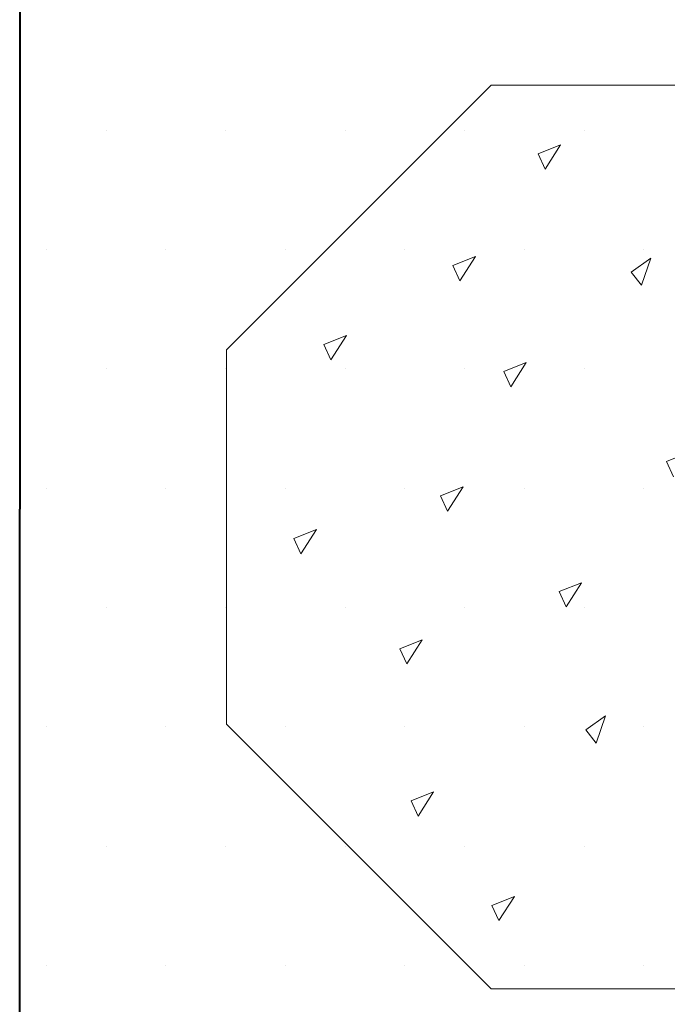
# Model space of a CAD drawing. Units: inches. Extents: x 459864 to 460310, y 324185 to 324787.
# Tile 4 of 112: x 460061.11 to 460069.72, y 324228.9 to 324241.99. Entities that reach past the tile are written whole.
import ezdxf

# ---------------------------------------------------------------- set-up
doc = ezdxf.new("R2010")
doc.units = ezdxf.units.IN
for name, color, linetype, lineweight in [('A-ANNO-DIMS', 2, 'Continuous', 18), ('A-WALL', 7, 'Continuous', 40), ('L-HRDS', 9, 'Continuous', 18), ('L-SITE-PATT', 252, 'Continuous', 13)]:
    doc.layers.add(name, color=color, linetype=linetype, lineweight=lineweight)
doc.styles.get("Standard").update_dxf_attribs({"font": 'arial.ttf'})
doc.dimstyles.new('ISO-25', dxfattribs={"dimtxt": 6, "dimasz": 2.5, "dimexe": 1.25, "dimexo": 0.625, "dimtad": 1, "dimdec": 1, "dimlunit": 3, "dimtxsty": 'Standard', "dimcen": 2.5, "dimadec": 0, "dimazin": 0, "dimtfac": 1, "dimtdec": 1, "dimtmove": 0, "dimatfit": 3, "dimfxl": 1, "dimarcsym": 0})

# ---------------------------------------------------------------- blocks, each defined once
blk = doc.blocks.new('Stepping Stone - hexagonal')
for p, q in [((-5.099, 10.067), (-10.964, 4.202)), ((3.195, 10.067), (-5.099, 10.067)), ((-3.564, 8.743), (-4.061, 8.544)), ((-3.906, 8.205), (-3.564, 8.743)), ((-4.061, 8.544), (-3.906, 8.205)), ((-5.451, 6.27), (-5.948, 6.072)), ((-5.793, 5.732), (-5.451, 6.27)), ((-1.567, 6.236), (-2.004, 5.927)), ((-1.775, 5.633), (-1.567, 6.236)), ((-5.948, 6.072), (-5.793, 5.732)), ((-2.004, 5.927), (-1.775, 5.633)), ((-8.308, 4.52), (-8.806, 4.321)), ((-8.651, 3.982), (-8.308, 4.52)), ((-10.964, 4.202), (-10.964, -4.092)), ((-8.806, 4.321), (-8.651, 3.982)), ((-4.324, 3.923), (-4.821, 3.724)), ((-4.821, 3.724), (-4.667, 3.385)), ((-4.667, 3.385), (-4.324, 3.923)), ((-0.723, 1.925), (-1.22, 1.726)), ((-1.22, 1.726), (-1.066, 1.387)), ((-5.724, 1.164), (-6.221, 0.965)), ((-6.066, 0.626), (-5.724, 1.164)), ((-6.221, 0.965), (-6.066, 0.626)), ((-8.972, 0.221), (-9.469, 0.023)), ((-9.314, -0.317), (-8.972, 0.221)), ((-9.469, 0.023), (-9.314, -0.317)), ((-3.099, -0.958), (-3.596, -1.157)), ((-3.441, -1.496), (-3.099, -0.958)), ((-3.596, -1.157), (-3.441, -1.496)), ((-6.63, -2.222), (-7.127, -2.421)), ((-6.972, -2.76), (-6.63, -2.222)), ((-7.127, -2.421), (-6.972, -2.76)), ((-2.567, -3.91), (-3.004, -4.219)), ((-2.774, -4.513), (-2.567, -3.91)), ((-10.964, -4.092), (-5.099, -9.957)), ((-3.004, -4.219), (-2.774, -4.513)), ((-6.377, -5.594), (-6.874, -5.792)), ((-6.719, -6.132), (-6.377, -5.594)), ((-6.874, -5.792), (-6.719, -6.132)), ((-4.588, -7.91), (-5.085, -8.109)), ((-4.93, -8.448), (-4.588, -7.91)), ((-5.085, -8.109), (-4.93, -8.448)), ((-5.099, -9.957), (3.195, -9.957))]:
    blk.add_line(p, q)
blk = doc.blocks.new('*D36')
at = {"layer": 'A-ANNO-DIMS', "color": 0, "lineweight": -2, "transparency": 16777216}
for p, q in [((460063.861, 324228.483), (460063.861, 324226.056)), ((460075.876, 324228.483), (460075.876, 324226.056)), ((460066.361, 324227.306), (460073.376, 324227.306)), ((460075.876, 324227.306), (460126.021, 324227.306))]:
    blk.add_line(p, q, dxfattribs=at)
at = {"layer": 'A-ANNO-DIMS', "color": 0, "transparency": 16777216}
for points in [[(460066.361, 324227.722), (460066.361, 324226.889), (460063.861, 324227.306)], [(460073.376, 324227.722), (460073.376, 324226.889), (460075.876, 324227.306)]]:
    blk.add_solid(points, dxfattribs=at)
at = {"layer": 'Defpoints', "color": 0, "transparency": 16777216}
for p in [(460063.861, 324229.108), (460075.876, 324229.108), (460075.876, 324227.306)]:
    blk.add_point(p, dxfattribs=at)
at = {"layer": 'A-ANNO-DIMS', "color": 0, "transparency": 16777216, "insert": (460102.199, 324230.994), "char_height": 6, "attachment_point": 5}
blk.add_mtext('PAVER 1\'-0"', dxfattribs=at)

msp = doc.modelspace()

# ---------------------------------------------------------------- hatches: boundary and pattern name
at = {"layer": 'L-SITE-PATT'}
h = msp.add_hatch(dxfattribs=at)
h.set_pattern_fill('DOTS', color=256)
h.paths.add_polyline_path([(460269.804, 324283.483), (460247.115, 324283.483), (460121.929, 324283.483), (460121.929, 324252.473), (460117.429, 324252.473), (460110.124, 324252.473), (460110.124, 324243.287), (460080.83, 324243.287), (460080.83, 324252.473), (460061.115, 324252.473), (460061.115, 324251.882), (460077.909, 324251.882), (460077.909, 324199.483), (460080.83, 324199.483), (460080.83, 324207.553), (460110.124, 324207.553), (460110.124, 324199.483), (460110.813, 324199.483), (460262.115, 324199.483), (460269.804, 324199.483)], flags=17)
edge = h.paths.add_edge_path(flags=0)
edge.add_ellipse((460222.59, 324263.813), major_axis=(-8.485, 8.485), ratio=1, start_angle=405, end_angle=495, ccw=False)
edge.add_line((460214.821, 324254.66), (460214.832, 324254.666))
edge.add_ellipse((460222.59, 324263.813), major_axis=(-8.485, 8.485), ratio=1, start_angle=405, end_angle=495, ccw=False)
edge.add_line((460210.759, 324261.781), (460210.768, 324261.787))
edge.add_ellipse((460222.59, 324263.813), major_axis=(-8.485, 8.485), ratio=1, start_angle=405, end_angle=495, ccw=False)
edge.add_ellipse((460222.59, 324263.813), major_axis=(-8.485, 8.485), ratio=1, start_angle=392.754, end_angle=405, ccw=False)
edge.add_ellipse((460222.59, 324263.813), major_axis=(-8.485, 8.485), ratio=1, start_angle=380.9347, end_angle=392.754, ccw=False)
edge.add_line((460211.337, 324267.985), (460211.34, 324267.985))
edge.add_ellipse((460222.59, 324263.813), major_axis=(-8.485, 8.485), ratio=1, start_angle=380.9347, end_angle=392.754, ccw=False)
edge.add_ellipse((460222.59, 324263.813), major_axis=(-8.485, 8.485), ratio=1, start_angle=347.9015, end_angle=380.9347, ccw=False)
edge.add_ellipse((460222.59, 324263.813), major_axis=(-8.485, 8.485), ratio=1, start_angle=327.0619, end_angle=347.9015, ccw=False)
edge.add_ellipse((460222.59, 324263.813), major_axis=(-8.485, 8.485), ratio=1, start_angle=278.3246, end_angle=327.0619, ccw=False)
edge.add_line((460225.158, 324275.536), (460225.158, 324275.535))
edge.add_ellipse((460222.59, 324263.813), major_axis=(-8.485, 8.485), ratio=1, start_angle=278.3246, end_angle=327.0619, ccw=False)
edge.add_ellipse((460222.59, 324263.813), major_axis=(-8.485, 8.485), ratio=1, start_angle=260.6436, end_angle=278.3246, ccw=False)
edge.add_ellipse((460222.59, 324263.813), major_axis=(-8.485, 8.485), ratio=1, start_angle=225, end_angle=260.6436, ccw=False)
edge.add_line((460234.509, 324265.243), (460234.501, 324265.239))
edge.add_ellipse((460222.59, 324263.813), major_axis=(-8.485, 8.485), ratio=1, start_angle=225, end_angle=260.6436, ccw=False)
edge.add_ellipse((460222.59, 324263.813), major_axis=(-8.485, 8.485), ratio=1, start_angle=495, end_angle=585, ccw=False)
edge.add_line((460234.437, 324261.861), (460234.424, 324261.858))
edge.add_ellipse((460222.59, 324263.813), major_axis=(-8.485, 8.485), ratio=1, start_angle=495, end_angle=585, ccw=False)
edge.add_line((460227.95, 324253.067), (460227.946, 324253.083))
edge.add_ellipse((460222.59, 324263.813), major_axis=(-8.485, 8.485), ratio=1, start_angle=495, end_angle=585, ccw=False)
edge.add_line((460226.223, 324252.369), (460226.211, 324252.38))
edge.add_ellipse((460222.59, 324263.813), major_axis=(-8.485, 8.485), ratio=1, start_angle=495, end_angle=585, ccw=False)
h.paths.add_polyline_path([(460219.651, 324254.347), (460218.461, 324253.545), (460218.275, 324254.789), (460219.642, 324256.542), (460219.625, 324260.848), (460216.11, 324257.333), (460214.35, 324256.978), (460215.416, 324259.356), (460212.524, 324258.496), (460213.137, 324259.93), (460218.507, 324263.813), (460222.59, 324263.813), (460222.59, 324267.807), (460218.176, 324272.212), (460219.026, 324274.639), (460222.59, 324272.811), (460222.59, 324275.423), (460223.057, 324274.825), (460222.675, 324273.492), (460225.912, 324267.135), (460219.625, 324260.848)], flags=0)
edge = h.paths.add_edge_path(flags=0)
edge.add_ellipse((460194.576, 324264.046), major_axis=(-8.485, 8.485), ratio=1, start_angle=495, end_angle=585, ccw=False)
edge.add_line((460199.936, 324253.3), (460199.932, 324253.316))
edge.add_ellipse((460194.576, 324264.046), major_axis=(-8.485, 8.485), ratio=1, start_angle=495, end_angle=585, ccw=False)
edge.add_line((460198.208, 324252.603), (460198.196, 324252.613))
edge.add_ellipse((460194.576, 324264.046), major_axis=(-8.485, 8.485), ratio=1, start_angle=495, end_angle=585, ccw=False)
edge.add_ellipse((460194.576, 324264.046), major_axis=(-8.485, 8.485), ratio=1, start_angle=405, end_angle=495, ccw=False)
edge.add_line((460186.806, 324254.893), (460186.817, 324254.899))
edge.add_ellipse((460194.576, 324264.046), major_axis=(-8.485, 8.485), ratio=1, start_angle=405, end_angle=495, ccw=False)
edge.add_line((460182.744, 324262.014), (460182.753, 324262.02))
edge.add_ellipse((460194.576, 324264.046), major_axis=(-8.485, 8.485), ratio=1, start_angle=405, end_angle=495, ccw=False)
edge.add_ellipse((460194.576, 324264.046), major_axis=(-8.485, 8.485), ratio=1, start_angle=392.754, end_angle=405, ccw=False)
edge.add_ellipse((460194.576, 324264.046), major_axis=(-8.485, 8.485), ratio=1, start_angle=380.9347, end_angle=392.754, ccw=False)
edge.add_line((460183.323, 324268.218), (460183.326, 324268.218))
edge.add_ellipse((460194.576, 324264.046), major_axis=(-8.485, 8.485), ratio=1, start_angle=380.9347, end_angle=392.754, ccw=False)
edge.add_ellipse((460194.576, 324264.046), major_axis=(-8.485, 8.485), ratio=1, start_angle=347.9015, end_angle=380.9347, ccw=False)
edge.add_ellipse((460194.576, 324264.046), major_axis=(-8.485, 8.485), ratio=1, start_angle=327.0619, end_angle=347.9015, ccw=False)
edge.add_ellipse((460194.576, 324264.046), major_axis=(-8.485, 8.485), ratio=1, start_angle=278.3246, end_angle=327.0619, ccw=False)
edge.add_line((460197.144, 324275.769), (460197.143, 324275.768))
edge.add_ellipse((460194.576, 324264.046), major_axis=(-8.485, 8.485), ratio=1, start_angle=278.3246, end_angle=327.0619, ccw=False)
edge.add_ellipse((460194.576, 324264.046), major_axis=(-8.485, 8.485), ratio=1, start_angle=260.6436, end_angle=278.3246, ccw=False)
edge.add_ellipse((460194.576, 324264.046), major_axis=(-8.485, 8.485), ratio=1, start_angle=225, end_angle=260.6436, ccw=False)
edge.add_line((460206.494, 324265.476), (460206.487, 324265.473))
edge.add_ellipse((460194.576, 324264.046), major_axis=(-8.485, 8.485), ratio=1, start_angle=225, end_angle=260.6436, ccw=False)
edge.add_ellipse((460194.576, 324264.046), major_axis=(-8.485, 8.485), ratio=1, start_angle=495, end_angle=585, ccw=False)
edge.add_line((460206.422, 324262.094), (460206.409, 324262.091))
h.paths.add_polyline_path([(460191.61, 324261.081), (460191.637, 324254.58), (460190.447, 324253.778), (460190.261, 324255.023), (460191.628, 324256.775), (460191.61, 324261.081), (460188.096, 324257.566), (460186.335, 324257.211), (460187.402, 324259.589), (460184.509, 324258.729), (460185.123, 324260.163), (460190.493, 324264.046), (460194.576, 324264.046), (460194.576, 324268.04), (460190.161, 324272.446), (460191.011, 324274.872), (460194.576, 324273.044), (460194.576, 324275.657), (460195.043, 324275.058), (460194.661, 324273.725), (460197.897, 324267.368)], flags=0)
edge = h.paths.add_edge_path(flags=0)
edge.add_ellipse((460252.912, 324263.578), major_axis=(-8.485, 8.485), ratio=1, start_angle=405, end_angle=495, ccw=False)
edge.add_line((460241.081, 324261.545), (460241.089, 324261.551))
edge.add_ellipse((460252.912, 324263.578), major_axis=(-8.485, 8.485), ratio=1, start_angle=405, end_angle=495, ccw=False)
edge.add_ellipse((460252.912, 324263.578), major_axis=(-8.485, 8.485), ratio=1, start_angle=392.754, end_angle=405, ccw=False)
edge.add_ellipse((460252.912, 324263.578), major_axis=(-8.485, 8.485), ratio=1, start_angle=380.9347, end_angle=392.754, ccw=False)
edge.add_line((460241.659, 324267.749), (460241.662, 324267.749))
edge.add_ellipse((460252.912, 324263.578), major_axis=(-8.485, 8.485), ratio=1, start_angle=380.9347, end_angle=392.754, ccw=False)
edge.add_ellipse((460252.912, 324263.578), major_axis=(-8.485, 8.485), ratio=1, start_angle=347.9015, end_angle=380.9347, ccw=False)
edge.add_ellipse((460252.912, 324263.578), major_axis=(-8.485, 8.485), ratio=1, start_angle=327.0619, end_angle=347.9015, ccw=False)
edge.add_ellipse((460252.912, 324263.578), major_axis=(-8.485, 8.485), ratio=1, start_angle=278.3246, end_angle=327.0619, ccw=False)
edge.add_line((460255.48, 324275.3), (460255.479, 324275.299))
edge.add_ellipse((460252.912, 324263.578), major_axis=(-8.485, 8.485), ratio=1, start_angle=278.3246, end_angle=327.0619, ccw=False)
edge.add_ellipse((460252.912, 324263.578), major_axis=(-8.485, 8.485), ratio=1, start_angle=260.6436, end_angle=278.3246, ccw=False)
edge.add_ellipse((460252.912, 324263.578), major_axis=(-8.485, 8.485), ratio=1, start_angle=225, end_angle=260.6436, ccw=False)
edge.add_line((460264.83, 324265.007), (460264.823, 324265.004))
edge.add_ellipse((460252.912, 324263.578), major_axis=(-8.485, 8.485), ratio=1, start_angle=225, end_angle=260.6436, ccw=False)
edge.add_ellipse((460252.912, 324263.578), major_axis=(-8.485, 8.485), ratio=1, start_angle=495, end_angle=585, ccw=False)
edge.add_line((460264.758, 324261.626), (460264.745, 324261.622))
edge.add_ellipse((460252.912, 324263.578), major_axis=(-8.485, 8.485), ratio=1, start_angle=495, end_angle=585, ccw=False)
edge.add_line((460258.272, 324252.832), (460258.268, 324252.848))
edge.add_ellipse((460252.912, 324263.578), major_axis=(-8.485, 8.485), ratio=1, start_angle=495, end_angle=585, ccw=False)
edge.add_line((460256.545, 324252.134), (460256.533, 324252.144))
edge.add_ellipse((460252.912, 324263.578), major_axis=(-8.485, 8.485), ratio=1, start_angle=495, end_angle=585, ccw=False)
edge.add_ellipse((460252.912, 324263.578), major_axis=(-8.485, 8.485), ratio=1, start_angle=405, end_angle=495, ccw=False)
edge.add_line((460245.143, 324254.424), (460245.153, 324254.43))
h.paths.add_polyline_path([(460244.672, 324256.742), (460245.738, 324259.12), (460242.846, 324258.26), (460243.459, 324259.694), (460248.829, 324263.578), (460252.912, 324263.578), (460252.912, 324267.571), (460248.497, 324271.977), (460249.348, 324274.403), (460252.912, 324272.576), (460252.912, 324275.188), (460253.379, 324274.589), (460252.997, 324273.257), (460256.233, 324266.899), (460249.946, 324260.612), (460249.973, 324254.111), (460248.783, 324253.309), (460248.597, 324254.554), (460249.964, 324256.306), (460249.946, 324260.612), (460246.432, 324257.097)], flags=0)
edge = h.paths.add_edge_path(flags=0)
edge.add_ellipse((460167.439, 324262.833), major_axis=(-8.485, 8.485), ratio=1, start_angle=495, end_angle=585, ccw=False)
edge.add_line((460172.799, 324252.087), (460172.795, 324252.103))
edge.add_ellipse((460167.439, 324262.833), major_axis=(-8.485, 8.485), ratio=1, start_angle=495, end_angle=585, ccw=False)
edge.add_line((460171.071, 324251.389), (460171.059, 324251.399))
edge.add_ellipse((460167.439, 324262.833), major_axis=(-8.485, 8.485), ratio=1, start_angle=495, end_angle=585, ccw=False)
edge.add_ellipse((460167.439, 324262.833), major_axis=(-8.485, 8.485), ratio=1, start_angle=405, end_angle=495, ccw=False)
edge.add_line((460159.669, 324253.679), (460159.68, 324253.685))
edge.add_ellipse((460167.439, 324262.833), major_axis=(-8.485, 8.485), ratio=1, start_angle=405, end_angle=495, ccw=False)
edge.add_line((460155.607, 324260.8), (460155.616, 324260.806))
edge.add_ellipse((460167.439, 324262.833), major_axis=(-8.485, 8.485), ratio=1, start_angle=405, end_angle=495, ccw=False)
edge.add_ellipse((460167.439, 324262.833), major_axis=(-8.485, 8.485), ratio=1, start_angle=392.754, end_angle=405, ccw=False)
edge.add_ellipse((460167.439, 324262.833), major_axis=(-8.485, 8.485), ratio=1, start_angle=380.9347, end_angle=392.754, ccw=False)
edge.add_line((460156.185, 324267.005), (460156.189, 324267.005))
edge.add_ellipse((460167.439, 324262.833), major_axis=(-8.485, 8.485), ratio=1, start_angle=380.9347, end_angle=392.754, ccw=False)
edge.add_ellipse((460167.439, 324262.833), major_axis=(-8.485, 8.485), ratio=1, start_angle=347.9015, end_angle=380.9347, ccw=False)
edge.add_ellipse((460167.439, 324262.833), major_axis=(-8.485, 8.485), ratio=1, start_angle=327.0619, end_angle=347.9015, ccw=False)
edge.add_ellipse((460167.439, 324262.833), major_axis=(-8.485, 8.485), ratio=1, start_angle=278.3246, end_angle=327.0619, ccw=False)
edge.add_line((460170.007, 324274.556), (460170.006, 324274.554))
edge.add_ellipse((460167.439, 324262.833), major_axis=(-8.485, 8.485), ratio=1, start_angle=278.3246, end_angle=327.0619, ccw=False)
edge.add_ellipse((460167.439, 324262.833), major_axis=(-8.485, 8.485), ratio=1, start_angle=260.6436, end_angle=278.3246, ccw=False)
edge.add_ellipse((460167.439, 324262.833), major_axis=(-8.485, 8.485), ratio=1, start_angle=225, end_angle=260.6436, ccw=False)
edge.add_line((460179.357, 324264.262), (460179.35, 324264.259))
edge.add_ellipse((460167.439, 324262.833), major_axis=(-8.485, 8.485), ratio=1, start_angle=225, end_angle=260.6436, ccw=False)
edge.add_ellipse((460167.439, 324262.833), major_axis=(-8.485, 8.485), ratio=1, start_angle=495, end_angle=585, ccw=False)
edge.add_line((460179.285, 324260.881), (460179.272, 324260.877))
h.paths.add_polyline_path([(460164.473, 324259.867), (460164.5, 324253.366), (460163.31, 324252.565), (460163.124, 324253.809), (460164.491, 324255.561), (460164.473, 324259.867), (460160.958, 324256.353), (460159.198, 324255.998), (460160.265, 324258.375), (460157.372, 324257.515), (460157.986, 324258.949), (460163.356, 324262.833), (460167.439, 324262.833), (460167.439, 324266.826), (460163.024, 324271.232), (460163.874, 324273.659), (460167.439, 324271.831), (460167.439, 324274.443), (460167.905, 324273.844), (460167.524, 324272.512), (460170.76, 324266.154)], flags=0)
edge = h.paths.add_edge_path(flags=0)
edge.add_ellipse((460140.758, 324262.37), major_axis=(-8.485, 8.485), ratio=1, start_angle=495, end_angle=585, ccw=False)
edge.add_line((460146.118, 324251.624), (460146.114, 324251.639))
edge.add_ellipse((460140.758, 324262.37), major_axis=(-8.485, 8.485), ratio=1, start_angle=495, end_angle=585, ccw=False)
edge.add_line((460144.391, 324250.926), (460144.379, 324250.936))
edge.add_ellipse((460140.758, 324262.37), major_axis=(-8.485, 8.485), ratio=1, start_angle=495, end_angle=585, ccw=False)
edge.add_ellipse((460140.758, 324262.37), major_axis=(-8.485, 8.485), ratio=1, start_angle=405, end_angle=495, ccw=False)
edge.add_line((460132.989, 324253.216), (460132.999, 324253.222))
edge.add_ellipse((460140.758, 324262.37), major_axis=(-8.485, 8.485), ratio=1, start_angle=405, end_angle=495, ccw=False)
edge.add_line((460128.927, 324260.337), (460128.935, 324260.343))
edge.add_ellipse((460140.758, 324262.37), major_axis=(-8.485, 8.485), ratio=1, start_angle=405, end_angle=495, ccw=False)
edge.add_ellipse((460140.758, 324262.37), major_axis=(-8.485, 8.485), ratio=1, start_angle=392.754, end_angle=405, ccw=False)
edge.add_ellipse((460140.758, 324262.37), major_axis=(-8.485, 8.485), ratio=1, start_angle=380.9347, end_angle=392.754, ccw=False)
edge.add_line((460129.505, 324266.541), (460129.508, 324266.541))
edge.add_ellipse((460140.758, 324262.37), major_axis=(-8.485, 8.485), ratio=1, start_angle=380.9347, end_angle=392.754, ccw=False)
edge.add_ellipse((460140.758, 324262.37), major_axis=(-8.485, 8.485), ratio=1, start_angle=347.9015, end_angle=380.9347, ccw=False)
edge.add_ellipse((460140.758, 324262.37), major_axis=(-8.485, 8.485), ratio=1, start_angle=327.0619, end_angle=347.9015, ccw=False)
edge.add_ellipse((460140.758, 324262.37), major_axis=(-8.485, 8.485), ratio=1, start_angle=278.3246, end_angle=327.0619, ccw=False)
edge.add_line((460143.326, 324274.092), (460143.325, 324274.091))
edge.add_ellipse((460140.758, 324262.37), major_axis=(-8.485, 8.485), ratio=1, start_angle=278.3246, end_angle=327.0619, ccw=False)
edge.add_ellipse((460140.758, 324262.37), major_axis=(-8.485, 8.485), ratio=1, start_angle=260.6436, end_angle=278.3246, ccw=False)
edge.add_ellipse((460140.758, 324262.37), major_axis=(-8.485, 8.485), ratio=1, start_angle=225, end_angle=260.6436, ccw=False)
edge.add_line((460152.677, 324263.799), (460152.669, 324263.796))
edge.add_ellipse((460140.758, 324262.37), major_axis=(-8.485, 8.485), ratio=1, start_angle=225, end_angle=260.6436, ccw=False)
edge.add_ellipse((460140.758, 324262.37), major_axis=(-8.485, 8.485), ratio=1, start_angle=495, end_angle=585, ccw=False)
edge.add_line((460152.604, 324260.418), (460152.592, 324260.414))
h.paths.add_polyline_path([(460137.792, 324259.404), (460137.819, 324252.903), (460136.629, 324252.101), (460136.443, 324253.346), (460137.81, 324255.098), (460137.792, 324259.404), (460134.278, 324255.889), (460132.518, 324255.534), (460133.584, 324257.912), (460130.692, 324257.052), (460131.305, 324258.486), (460136.675, 324262.37), (460140.758, 324262.37), (460140.758, 324266.363), (460136.343, 324270.769), (460137.194, 324273.195), (460140.758, 324271.367), (460140.758, 324273.98), (460141.225, 324273.381), (460140.843, 324272.049), (460144.079, 324265.691)], flags=0)
h.paths.add_polyline_path([(460110.124, 324227.414), (460080.83, 324227.414), (460080.83, 324235.484), (460110.124, 324235.484)], flags=16)
h.paths.add_polyline_path([(460110.124, 324220.797), (460110.124, 324212.727), (460080.83, 324212.727), (460080.83, 324220.797)], flags=16)
h.paths.add_polyline_path([(460269.804, 324283.483), (460247.115, 324283.483), (460121.929, 324283.483), (460121.929, 324252.473), (460117.429, 324252.473), (460110.124, 324252.473), (460110.124, 324243.287), (460080.83, 324243.287), (460080.83, 324252.473), (460061.115, 324252.473), (460061.115, 324251.882), (460077.909, 324251.882), (460077.909, 324199.483), (460080.83, 324199.483), (460080.83, 324207.553), (460110.124, 324207.553), (460110.124, 324199.483), (460262.115, 324199.483), (460269.804, 324199.483)], flags=17)
h.paths.add_polyline_path([(460219.651, 324254.347), (460218.461, 324253.545), (460218.275, 324254.789), (460219.642, 324256.542), (460219.625, 324260.848), (460216.11, 324257.333), (460214.35, 324256.978), (460215.416, 324259.356), (460212.524, 324258.496), (460213.137, 324259.93), (460218.507, 324263.813), (460222.59, 324263.813), (460220.18, 324266.223), (460215.461, 324265.308), (460211.835, 324266.137), (460216.247, 324267.985), (460218.418, 324267.985), (460222.59, 324263.813), (460222.59, 324267.807), (460218.176, 324272.212), (460219.026, 324274.639), (460222.59, 324272.811), (460222.59, 324275.423), (460223.057, 324274.825), (460222.675, 324273.492), (460225.912, 324267.135), (460222.59, 324263.813), (460231.383, 324263.813), (460228.485, 324262.488), (460224.425, 324261.978), (460228.68, 324257.724), (460228.966, 324254.791), (460227.142, 324256.537), (460227.542, 324254.819), (460227.333, 324253.614), (460222.59, 324259.985), (460222.59, 324255.497), (460221.377, 324256.541), (460220.576, 324261.799), (460219.625, 324260.848)], flags=0)
h.paths.add_polyline_path([(460199.127, 324256.77), (460199.528, 324255.052), (460199.319, 324253.848), (460194.576, 324260.218), (460194.576, 324255.73), (460193.363, 324256.774), (460192.561, 324262.032), (460191.61, 324261.081), (460191.637, 324254.58), (460190.447, 324253.778), (460190.261, 324255.023), (460191.628, 324256.775), (460191.61, 324261.081), (460188.096, 324257.566), (460186.335, 324257.211), (460187.402, 324259.589), (460184.509, 324258.729), (460185.123, 324260.163), (460190.493, 324264.046), (460194.576, 324264.046), (460192.166, 324266.456), (460187.446, 324265.541), (460183.82, 324266.37), (460188.232, 324268.218), (460190.404, 324268.218), (460194.576, 324264.046), (460194.576, 324268.04), (460190.161, 324272.446), (460191.011, 324274.872), (460194.576, 324273.044), (460194.576, 324275.657), (460195.043, 324275.058), (460194.661, 324273.725), (460197.897, 324267.368), (460194.576, 324264.046), (460203.368, 324264.046), (460200.47, 324262.721), (460196.411, 324262.212), (460200.665, 324257.957), (460200.951, 324255.024)], flags=0)
h.paths.add_polyline_path([(460244.672, 324256.742), (460245.738, 324259.12), (460242.846, 324258.26), (460243.459, 324259.694), (460248.829, 324263.578), (460252.912, 324263.578), (460250.502, 324265.987), (460245.783, 324265.072), (460242.156, 324265.901), (460246.568, 324267.749), (460248.74, 324267.749), (460252.912, 324263.578), (460252.912, 324267.571), (460248.497, 324271.977), (460249.348, 324274.403), (460252.912, 324272.576), (460252.912, 324275.188), (460253.379, 324274.589), (460252.997, 324273.257), (460256.233, 324266.899), (460252.912, 324263.578), (460261.705, 324263.578), (460258.806, 324262.252), (460254.747, 324261.743), (460259.002, 324257.488), (460259.288, 324254.555), (460257.463, 324256.301), (460257.864, 324254.583), (460257.655, 324253.379), (460252.912, 324259.749), (460252.912, 324255.261), (460251.699, 324256.305), (460250.897, 324261.563), (460249.946, 324260.612), (460249.973, 324254.111), (460248.783, 324253.309), (460248.597, 324254.554), (460249.964, 324256.306), (460249.946, 324260.612), (460246.432, 324257.097)], flags=0)
h.paths.add_polyline_path([(460173.528, 324256.743), (460173.814, 324253.811), (460171.99, 324255.556), (460172.39, 324253.838), (460172.182, 324252.634), (460167.439, 324259.004), (460167.439, 324254.516), (460166.226, 324255.56), (460165.424, 324260.818), (460164.473, 324259.867), (460164.5, 324253.366), (460163.31, 324252.565), (460163.124, 324253.809), (460164.491, 324255.561), (460164.473, 324259.867), (460160.958, 324256.353), (460159.198, 324255.998), (460160.265, 324258.375), (460157.372, 324257.515), (460157.986, 324258.949), (460163.356, 324262.833), (460167.439, 324262.833), (460165.029, 324265.243), (460160.309, 324264.327), (460156.683, 324265.156), (460161.095, 324267.005), (460163.267, 324267.005), (460167.439, 324262.833), (460167.439, 324266.826), (460163.024, 324271.232), (460163.874, 324273.659), (460167.439, 324271.831), (460167.439, 324274.443), (460167.905, 324273.844), (460167.524, 324272.512), (460170.76, 324266.154), (460167.439, 324262.833), (460176.231, 324262.833), (460173.333, 324261.507), (460169.274, 324260.998)], flags=0)
h.paths.add_polyline_path([(460146.848, 324256.28), (460147.134, 324253.347), (460145.31, 324255.093), (460145.71, 324253.375), (460145.501, 324252.171), (460140.758, 324258.541), (460140.758, 324254.053), (460139.545, 324255.097), (460138.744, 324260.355), (460137.792, 324259.404), (460137.819, 324252.903), (460136.629, 324252.101), (460136.443, 324253.346), (460137.81, 324255.098), (460137.792, 324259.404), (460134.278, 324255.889), (460132.518, 324255.534), (460133.584, 324257.912), (460130.692, 324257.052), (460131.305, 324258.486), (460136.675, 324262.37), (460140.758, 324262.37), (460138.348, 324264.779), (460133.629, 324263.864), (460130.002, 324264.693), (460134.414, 324266.541), (460136.586, 324266.541), (460140.758, 324262.37), (460140.758, 324266.363), (460136.343, 324270.769), (460137.194, 324273.195), (460140.758, 324271.367), (460140.758, 324273.98), (460141.225, 324273.381), (460140.843, 324272.049), (460144.079, 324265.691), (460140.758, 324262.37), (460149.551, 324262.37), (460146.653, 324261.044), (460142.593, 324260.535)], flags=0)
edge = h.paths.add_edge_path()
edge.add_line((460269.804, 324272.549), (460260.881, 324272.549))
edge.add_ellipse((460252.912, 324263.578), major_axis=(-8.485, 8.485), ratio=1, start_angle=260.6436, end_angle=273.3846, ccw=False)
edge.add_line((460262.283, 324271.092), (460262.261, 324271.091))
edge.add_ellipse((460252.912, 324263.578), major_axis=(-8.485, 8.485), ratio=1, start_angle=260.6436, end_angle=273.3846, ccw=False)
edge.add_ellipse((460252.912, 324263.578), major_axis=(-8.485, 8.485), ratio=1, start_angle=225, end_angle=260.6436, ccw=False)
edge.add_line((460263.609, 324269.063), (460263.572, 324269.058))
edge.add_ellipse((460252.912, 324263.578), major_axis=(-8.485, 8.485), ratio=1, start_angle=225, end_angle=260.6436, ccw=False)
edge.add_line((460264.615, 324266.306), (460264.585, 324266.305))
edge.add_ellipse((460252.912, 324263.578), major_axis=(-8.485, 8.485), ratio=1, start_angle=225, end_angle=260.6436, ccw=False)
edge.add_line((460264.83, 324265.007), (460264.823, 324265.004))
edge.add_ellipse((460252.912, 324263.578), major_axis=(-8.485, 8.485), ratio=1, start_angle=225, end_angle=260.6436, ccw=False)
edge.add_ellipse((460252.912, 324263.578), major_axis=(-8.485, 8.485), ratio=1, start_angle=495, end_angle=585, ccw=False)
edge.add_line((460264.758, 324261.626), (460264.745, 324261.622))
edge.add_ellipse((460252.912, 324263.578), major_axis=(-8.485, 8.485), ratio=1, start_angle=495, end_angle=585, ccw=False)
edge.add_line((460263.442, 324257.739), (460263.389, 324257.779))
edge.add_ellipse((460252.912, 324263.578), major_axis=(-8.485, 8.485), ratio=1, start_angle=495, end_angle=585, ccw=False)
edge.add_line((460258.128, 324252.744), (460258.102, 324252.779))
edge.add_ellipse((460252.912, 324263.578), major_axis=(-8.485, 8.485), ratio=1, start_angle=495, end_angle=585, ccw=False)
edge.add_line((460256.545, 324252.134), (460256.533, 324252.144))
edge.add_ellipse((460252.912, 324263.578), major_axis=(-8.485, 8.485), ratio=1, start_angle=495, end_angle=585, ccw=False)
edge.add_ellipse((460252.912, 324263.578), major_axis=(-8.485, 8.485), ratio=1, start_angle=405, end_angle=495, ccw=False)
edge.add_line((460250.594, 324251.78), (460250.605, 324251.82))
edge.add_ellipse((460252.912, 324263.578), major_axis=(-8.485, 8.485), ratio=1, start_angle=405, end_angle=495, ccw=False)
edge.add_line((460245.143, 324254.424), (460245.153, 324254.43))
edge.add_ellipse((460252.912, 324263.578), major_axis=(-8.485, 8.485), ratio=1, start_angle=405, end_angle=495, ccw=False)
edge.add_line((460243.525, 324256.059), (460243.56, 324256.091))
edge.add_ellipse((460252.912, 324263.578), major_axis=(-8.485, 8.485), ratio=1, start_angle=405, end_angle=495, ccw=False)
edge.add_line((460241.44, 324259.893), (460241.522, 324259.896))
edge.add_ellipse((460252.912, 324263.578), major_axis=(-8.485, 8.485), ratio=1, start_angle=405, end_angle=495, ccw=False)
edge.add_line((460241.081, 324261.545), (460241.089, 324261.551))
edge.add_ellipse((460252.912, 324263.578), major_axis=(-8.485, 8.485), ratio=1, start_angle=405, end_angle=495, ccw=False)
edge.add_ellipse((460252.912, 324263.578), major_axis=(-8.485, 8.485), ratio=1, start_angle=392.754, end_angle=405, ccw=False)
edge.add_line((460241.05, 324265.438), (460241.063, 324265.443))
edge.add_ellipse((460252.912, 324263.578), major_axis=(-8.485, 8.485), ratio=1, start_angle=392.754, end_angle=405, ccw=False)
edge.add_ellipse((460252.912, 324263.578), major_axis=(-8.485, 8.485), ratio=1, start_angle=380.9347, end_angle=392.754, ccw=False)
edge.add_line((460241.452, 324267.176), (460241.469, 324267.171))
edge.add_ellipse((460252.912, 324263.578), major_axis=(-8.485, 8.485), ratio=1, start_angle=380.9347, end_angle=392.754, ccw=False)
edge.add_line((460241.659, 324267.749), (460241.662, 324267.749))
edge.add_ellipse((460252.912, 324263.578), major_axis=(-8.485, 8.485), ratio=1, start_angle=380.9347, end_angle=392.754, ccw=False)
edge.add_ellipse((460252.912, 324263.578), major_axis=(-8.485, 8.485), ratio=1, start_angle=356.6154, end_angle=380.9347, ccw=False)
edge.add_line((460244.88, 324272.488), (460244.713, 324272.549))
edge.add_line((460244.713, 324272.549), (460230.817, 324272.549))
edge.add_ellipse((460222.59, 324263.813), major_axis=(-8.485, 8.485), ratio=1, start_angle=260.6436, end_angle=271.7178, ccw=False)
edge.add_ellipse((460222.59, 324263.813), major_axis=(-8.485, 8.485), ratio=1, start_angle=225, end_angle=260.6436, ccw=False)
edge.add_line((460233.287, 324269.299), (460233.25, 324269.294))
edge.add_ellipse((460222.59, 324263.813), major_axis=(-8.485, 8.485), ratio=1, start_angle=225, end_angle=260.6436, ccw=False)
edge.add_line((460234.294, 324266.541), (460234.264, 324266.541))
edge.add_ellipse((460222.59, 324263.813), major_axis=(-8.485, 8.485), ratio=1, start_angle=225, end_angle=260.6436, ccw=False)
edge.add_line((460234.509, 324265.243), (460234.501, 324265.239))
edge.add_ellipse((460222.59, 324263.813), major_axis=(-8.485, 8.485), ratio=1, start_angle=225, end_angle=260.6436, ccw=False)
edge.add_ellipse((460222.59, 324263.813), major_axis=(-8.485, 8.485), ratio=1, start_angle=495, end_angle=585, ccw=False)
edge.add_line((460234.437, 324261.861), (460234.424, 324261.858))
edge.add_ellipse((460222.59, 324263.813), major_axis=(-8.485, 8.485), ratio=1, start_angle=495, end_angle=585, ccw=False)
edge.add_line((460233.121, 324257.975), (460233.068, 324258.015))
edge.add_ellipse((460222.59, 324263.813), major_axis=(-8.485, 8.485), ratio=1, start_angle=495, end_angle=585, ccw=False)
edge.add_line((460227.806, 324252.979), (460227.78, 324253.014))
edge.add_ellipse((460222.59, 324263.813), major_axis=(-8.485, 8.485), ratio=1, start_angle=495, end_angle=585, ccw=False)
edge.add_line((460226.223, 324252.369), (460226.211, 324252.38))
edge.add_ellipse((460222.59, 324263.813), major_axis=(-8.485, 8.485), ratio=1, start_angle=495, end_angle=585, ccw=False)
edge.add_ellipse((460222.59, 324263.813), major_axis=(-8.485, 8.485), ratio=1, start_angle=405, end_angle=495, ccw=False)
edge.add_line((460220.272, 324252.016), (460220.283, 324252.055))
edge.add_ellipse((460222.59, 324263.813), major_axis=(-8.485, 8.485), ratio=1, start_angle=405, end_angle=495, ccw=False)
edge.add_line((460214.821, 324254.66), (460214.832, 324254.666))
edge.add_ellipse((460222.59, 324263.813), major_axis=(-8.485, 8.485), ratio=1, start_angle=405, end_angle=495, ccw=False)
edge.add_line((460213.203, 324256.295), (460213.239, 324256.327))
edge.add_ellipse((460222.59, 324263.813), major_axis=(-8.485, 8.485), ratio=1, start_angle=405, end_angle=495, ccw=False)
edge.add_line((460211.118, 324260.128), (460211.201, 324260.131))
edge.add_ellipse((460222.59, 324263.813), major_axis=(-8.485, 8.485), ratio=1, start_angle=405, end_angle=495, ccw=False)
edge.add_line((460210.759, 324261.781), (460210.768, 324261.787))
edge.add_ellipse((460222.59, 324263.813), major_axis=(-8.485, 8.485), ratio=1, start_angle=405, end_angle=495, ccw=False)
edge.add_ellipse((460222.59, 324263.813), major_axis=(-8.485, 8.485), ratio=1, start_angle=392.754, end_angle=405, ccw=False)
edge.add_line((460210.729, 324265.673), (460210.741, 324265.678))
edge.add_ellipse((460222.59, 324263.813), major_axis=(-8.485, 8.485), ratio=1, start_angle=392.754, end_angle=405, ccw=False)
edge.add_ellipse((460222.59, 324263.813), major_axis=(-8.485, 8.485), ratio=1, start_angle=380.9347, end_angle=392.754, ccw=False)
edge.add_line((460211.13, 324267.412), (460211.147, 324267.407))
edge.add_ellipse((460222.59, 324263.813), major_axis=(-8.485, 8.485), ratio=1, start_angle=380.9347, end_angle=392.754, ccw=False)
edge.add_line((460211.337, 324267.985), (460211.34, 324267.985))
edge.add_ellipse((460222.59, 324263.813), major_axis=(-8.485, 8.485), ratio=1, start_angle=380.9347, end_angle=392.754, ccw=False)
edge.add_ellipse((460222.59, 324263.813), major_axis=(-8.485, 8.485), ratio=1, start_angle=358.2822, end_angle=380.9347, ccw=False)
edge.add_line((460213.705, 324271.902), (460213.709, 324271.869))
edge.add_ellipse((460222.59, 324263.813), major_axis=(-8.485, 8.485), ratio=1, start_angle=358.2822, end_angle=380.9347, ccw=False)
edge.add_line((460214.363, 324272.549), (460203.078, 324272.549))
edge.add_line((460203.078, 324272.549), (460203.06, 324272.531))
edge.add_ellipse((460194.576, 324264.046), major_axis=(-8.485, 8.485), ratio=1, start_angle=260.6436, end_angle=270.1168, ccw=False)
edge.add_line((460203.957, 324271.561), (460203.921, 324271.56))
edge.add_ellipse((460194.576, 324264.046), major_axis=(-8.485, 8.485), ratio=1, start_angle=260.6436, end_angle=270.1168, ccw=False)
edge.add_ellipse((460194.576, 324264.046), major_axis=(-8.485, 8.485), ratio=1, start_angle=225, end_angle=260.6436, ccw=False)
edge.add_line((460205.272, 324269.532), (460205.235, 324269.527))
edge.add_ellipse((460194.576, 324264.046), major_axis=(-8.485, 8.485), ratio=1, start_angle=225, end_angle=260.6436, ccw=False)
edge.add_line((460206.279, 324266.774), (460206.249, 324266.774))
edge.add_ellipse((460194.576, 324264.046), major_axis=(-8.485, 8.485), ratio=1, start_angle=225, end_angle=260.6436, ccw=False)
edge.add_line((460206.494, 324265.476), (460206.487, 324265.473))
edge.add_ellipse((460194.576, 324264.046), major_axis=(-8.485, 8.485), ratio=1, start_angle=225, end_angle=260.6436, ccw=False)
edge.add_ellipse((460194.576, 324264.046), major_axis=(-8.485, 8.485), ratio=1, start_angle=495, end_angle=585, ccw=False)
edge.add_line((460206.422, 324262.094), (460206.409, 324262.091))
edge.add_ellipse((460194.576, 324264.046), major_axis=(-8.485, 8.485), ratio=1, start_angle=495, end_angle=585, ccw=False)
edge.add_line((460205.106, 324258.208), (460205.053, 324258.248))
edge.add_ellipse((460194.576, 324264.046), major_axis=(-8.485, 8.485), ratio=1, start_angle=495, end_angle=585, ccw=False)
edge.add_line((460199.792, 324253.212), (460199.766, 324253.248))
edge.add_ellipse((460194.576, 324264.046), major_axis=(-8.485, 8.485), ratio=1, start_angle=495, end_angle=585, ccw=False)
edge.add_line((460198.208, 324252.603), (460198.196, 324252.613))
edge.add_ellipse((460194.576, 324264.046), major_axis=(-8.485, 8.485), ratio=1, start_angle=495, end_angle=585, ccw=False)
edge.add_ellipse((460194.576, 324264.046), major_axis=(-8.485, 8.485), ratio=1, start_angle=405, end_angle=495, ccw=False)
edge.add_line((460192.258, 324252.249), (460192.268, 324252.289))
edge.add_ellipse((460194.576, 324264.046), major_axis=(-8.485, 8.485), ratio=1, start_angle=405, end_angle=495, ccw=False)
edge.add_line((460186.806, 324254.893), (460186.817, 324254.899))
edge.add_ellipse((460194.576, 324264.046), major_axis=(-8.485, 8.485), ratio=1, start_angle=405, end_angle=495, ccw=False)
edge.add_line((460185.188, 324256.528), (460185.224, 324256.56))
edge.add_ellipse((460194.576, 324264.046), major_axis=(-8.485, 8.485), ratio=1, start_angle=405, end_angle=495, ccw=False)
edge.add_line((460183.104, 324260.362), (460183.186, 324260.365))
edge.add_ellipse((460194.576, 324264.046), major_axis=(-8.485, 8.485), ratio=1, start_angle=405, end_angle=495, ccw=False)
edge.add_line((460182.744, 324262.014), (460182.753, 324262.02))
edge.add_ellipse((460194.576, 324264.046), major_axis=(-8.485, 8.485), ratio=1, start_angle=405, end_angle=495, ccw=False)
edge.add_ellipse((460194.576, 324264.046), major_axis=(-8.485, 8.485), ratio=1, start_angle=392.754, end_angle=405, ccw=False)
edge.add_line((460182.714, 324265.906), (460182.726, 324265.912))
edge.add_ellipse((460194.576, 324264.046), major_axis=(-8.485, 8.485), ratio=1, start_angle=392.754, end_angle=405, ccw=False)
edge.add_ellipse((460194.576, 324264.046), major_axis=(-8.485, 8.485), ratio=1, start_angle=380.9347, end_angle=392.754, ccw=False)
edge.add_line((460183.116, 324267.645), (460183.133, 324267.64))
edge.add_ellipse((460194.576, 324264.046), major_axis=(-8.485, 8.485), ratio=1, start_angle=380.9347, end_angle=392.754, ccw=False)
edge.add_line((460183.323, 324268.218), (460183.326, 324268.218))
edge.add_ellipse((460194.576, 324264.046), major_axis=(-8.485, 8.485), ratio=1, start_angle=380.9347, end_angle=392.754, ccw=False)
edge.add_ellipse((460194.576, 324264.046), major_axis=(-8.485, 8.485), ratio=1, start_angle=359.8832, end_angle=380.9347, ccw=False)
edge.add_line((460184.491, 324270.611), (460184.553, 324270.611))
edge.add_ellipse((460194.576, 324264.046), major_axis=(-8.485, 8.485), ratio=1, start_angle=359.8832, end_angle=380.9347, ccw=False)
edge.add_line((460185.346, 324271.76), (460185.379, 324271.728))
edge.add_ellipse((460194.576, 324264.046), major_axis=(-8.485, 8.485), ratio=1, start_angle=359.8832, end_angle=380.9347, ccw=False)
edge.add_line((460185.697, 324272.086), (460185.633, 324272.549))
edge.add_line((460185.633, 324272.549), (460174.683, 324272.549))
edge.add_line((460174.683, 324272.549), (460174.606, 324272.457))
edge.add_ellipse((460167.439, 324262.833), major_axis=(-8.485, 8.485), ratio=1, start_angle=260.6436, end_angle=278.3246, ccw=False)
edge.add_ellipse((460167.439, 324262.833), major_axis=(-8.485, 8.485), ratio=1, start_angle=225, end_angle=260.6436, ccw=False)
edge.add_line((460178.135, 324268.318), (460178.098, 324268.313))
edge.add_ellipse((460167.439, 324262.833), major_axis=(-8.485, 8.485), ratio=1, start_angle=225, end_angle=260.6436, ccw=False)
edge.add_line((460179.142, 324265.561), (460179.112, 324265.56))
edge.add_ellipse((460167.439, 324262.833), major_axis=(-8.485, 8.485), ratio=1, start_angle=225, end_angle=260.6436, ccw=False)
edge.add_line((460179.357, 324264.262), (460179.35, 324264.259))
edge.add_ellipse((460167.439, 324262.833), major_axis=(-8.485, 8.485), ratio=1, start_angle=225, end_angle=260.6436, ccw=False)
edge.add_ellipse((460167.439, 324262.833), major_axis=(-8.485, 8.485), ratio=1, start_angle=495, end_angle=585, ccw=False)
edge.add_line((460179.285, 324260.881), (460179.272, 324260.877))
edge.add_ellipse((460167.439, 324262.833), major_axis=(-8.485, 8.485), ratio=1, start_angle=495, end_angle=585, ccw=False)
edge.add_line((460177.969, 324256.994), (460177.916, 324257.034))
edge.add_ellipse((460167.439, 324262.833), major_axis=(-8.485, 8.485), ratio=1, start_angle=495, end_angle=585, ccw=False)
edge.add_line((460172.655, 324251.999), (460172.629, 324252.034))
edge.add_ellipse((460167.439, 324262.833), major_axis=(-8.485, 8.485), ratio=1, start_angle=495, end_angle=585, ccw=False)
edge.add_line((460171.071, 324251.389), (460171.059, 324251.399))
edge.add_ellipse((460167.439, 324262.833), major_axis=(-8.485, 8.485), ratio=1, start_angle=495, end_angle=585, ccw=False)
edge.add_ellipse((460167.439, 324262.833), major_axis=(-8.485, 8.485), ratio=1, start_angle=405, end_angle=495, ccw=False)
edge.add_line((460165.121, 324251.036), (460165.131, 324251.075))
edge.add_ellipse((460167.439, 324262.833), major_axis=(-8.485, 8.485), ratio=1, start_angle=405, end_angle=495, ccw=False)
edge.add_line((460159.669, 324253.679), (460159.68, 324253.685))
edge.add_ellipse((460167.439, 324262.833), major_axis=(-8.485, 8.485), ratio=1, start_angle=405, end_angle=495, ccw=False)
edge.add_line((460158.051, 324255.314), (460158.087, 324255.347))
edge.add_ellipse((460167.439, 324262.833), major_axis=(-8.485, 8.485), ratio=1, start_angle=405, end_angle=495, ccw=False)
edge.add_line((460155.967, 324259.148), (460156.049, 324259.151))
edge.add_ellipse((460167.439, 324262.833), major_axis=(-8.485, 8.485), ratio=1, start_angle=405, end_angle=495, ccw=False)
edge.add_line((460155.607, 324260.8), (460155.616, 324260.806))
edge.add_ellipse((460167.439, 324262.833), major_axis=(-8.485, 8.485), ratio=1, start_angle=405, end_angle=495, ccw=False)
edge.add_ellipse((460167.439, 324262.833), major_axis=(-8.485, 8.485), ratio=1, start_angle=392.754, end_angle=405, ccw=False)
edge.add_line((460155.577, 324264.693), (460155.589, 324264.698))
edge.add_ellipse((460167.439, 324262.833), major_axis=(-8.485, 8.485), ratio=1, start_angle=392.754, end_angle=405, ccw=False)
edge.add_ellipse((460167.439, 324262.833), major_axis=(-8.485, 8.485), ratio=1, start_angle=380.9347, end_angle=392.754, ccw=False)
edge.add_line((460155.979, 324266.432), (460155.996, 324266.426))
edge.add_ellipse((460167.439, 324262.833), major_axis=(-8.485, 8.485), ratio=1, start_angle=380.9347, end_angle=392.754, ccw=False)
edge.add_line((460156.185, 324267.005), (460156.189, 324267.005))
edge.add_ellipse((460167.439, 324262.833), major_axis=(-8.485, 8.485), ratio=1, start_angle=380.9347, end_angle=392.754, ccw=False)
edge.add_ellipse((460167.439, 324262.833), major_axis=(-8.485, 8.485), ratio=1, start_angle=350.9345, end_angle=380.9347, ccw=False)
edge.add_line((460157.363, 324269.397), (460157.414, 324269.397))
edge.add_ellipse((460167.439, 324262.833), major_axis=(-8.485, 8.485), ratio=1, start_angle=350.9345, end_angle=380.9347, ccw=False)
edge.add_line((460158.221, 324270.535), (460158.236, 324270.519))
edge.add_ellipse((460167.439, 324262.833), major_axis=(-8.485, 8.485), ratio=1, start_angle=350.9345, end_angle=380.9347, ccw=False)
edge.add_line((460159.379, 324271.753), (460159.419, 324271.738))
edge.add_ellipse((460167.439, 324262.833), major_axis=(-8.485, 8.485), ratio=1, start_angle=350.9345, end_angle=380.9347, ccw=False)
edge.add_line((460160.396, 324272.549), (460147.112, 324272.549))
edge.add_ellipse((460140.758, 324262.37), major_axis=(-8.485, 8.485), ratio=1, start_angle=278.3246, end_angle=283.0261, ccw=False)
edge.add_ellipse((460140.758, 324262.37), major_axis=(-8.485, 8.485), ratio=1, start_angle=260.6436, end_angle=278.3246, ccw=False)
edge.add_ellipse((460140.758, 324262.37), major_axis=(-8.485, 8.485), ratio=1, start_angle=225, end_angle=260.6436, ccw=False)
edge.add_line((460151.455, 324267.855), (460151.418, 324267.85))
edge.add_ellipse((460140.758, 324262.37), major_axis=(-8.485, 8.485), ratio=1, start_angle=225, end_angle=260.6436, ccw=False)
edge.add_line((460152.462, 324265.098), (460152.431, 324265.097))
edge.add_ellipse((460140.758, 324262.37), major_axis=(-8.485, 8.485), ratio=1, start_angle=225, end_angle=260.6436, ccw=False)
edge.add_line((460152.677, 324263.799), (460152.669, 324263.796))
edge.add_ellipse((460140.758, 324262.37), major_axis=(-8.485, 8.485), ratio=1, start_angle=225, end_angle=260.6436, ccw=False)
edge.add_ellipse((460140.758, 324262.37), major_axis=(-8.485, 8.485), ratio=1, start_angle=495, end_angle=585, ccw=False)
edge.add_line((460152.604, 324260.418), (460152.592, 324260.414))
edge.add_ellipse((460140.758, 324262.37), major_axis=(-8.485, 8.485), ratio=1, start_angle=495, end_angle=585, ccw=False)
edge.add_line((460151.288, 324256.531), (460151.235, 324256.571))
edge.add_ellipse((460140.758, 324262.37), major_axis=(-8.485, 8.485), ratio=1, start_angle=495, end_angle=585, ccw=False)
edge.add_line((460145.974, 324251.535), (460145.948, 324251.571))
edge.add_ellipse((460140.758, 324262.37), major_axis=(-8.485, 8.485), ratio=1, start_angle=495, end_angle=585, ccw=False)
edge.add_line((460144.391, 324250.926), (460144.379, 324250.936))
edge.add_ellipse((460140.758, 324262.37), major_axis=(-8.485, 8.485), ratio=1, start_angle=495, end_angle=585, ccw=False)
edge.add_ellipse((460140.758, 324262.37), major_axis=(-8.485, 8.485), ratio=1, start_angle=405, end_angle=495, ccw=False)
edge.add_line((460138.44, 324250.572), (460138.451, 324250.612))
edge.add_ellipse((460140.758, 324262.37), major_axis=(-8.485, 8.485), ratio=1, start_angle=405, end_angle=495, ccw=False)
edge.add_line((460132.989, 324253.216), (460132.999, 324253.222))
edge.add_ellipse((460140.758, 324262.37), major_axis=(-8.485, 8.485), ratio=1, start_angle=405, end_angle=495, ccw=False)
edge.add_line((460131.371, 324254.851), (460131.406, 324254.883))
edge.add_ellipse((460140.758, 324262.37), major_axis=(-8.485, 8.485), ratio=1, start_angle=405, end_angle=495, ccw=False)
edge.add_line((460129.286, 324258.685), (460129.369, 324258.688))
edge.add_ellipse((460140.758, 324262.37), major_axis=(-8.485, 8.485), ratio=1, start_angle=405, end_angle=495, ccw=False)
edge.add_line((460128.927, 324260.337), (460128.935, 324260.343))
edge.add_ellipse((460140.758, 324262.37), major_axis=(-8.485, 8.485), ratio=1, start_angle=405, end_angle=495, ccw=False)
edge.add_ellipse((460140.758, 324262.37), major_axis=(-8.485, 8.485), ratio=1, start_angle=392.754, end_angle=405, ccw=False)
edge.add_line((460128.896, 324264.23), (460128.909, 324264.235))
edge.add_ellipse((460140.758, 324262.37), major_axis=(-8.485, 8.485), ratio=1, start_angle=392.754, end_angle=405, ccw=False)
edge.add_ellipse((460140.758, 324262.37), major_axis=(-8.485, 8.485), ratio=1, start_angle=380.9347, end_angle=392.754, ccw=False)
edge.add_line((460129.298, 324265.968), (460129.315, 324265.963))
edge.add_ellipse((460140.758, 324262.37), major_axis=(-8.485, 8.485), ratio=1, start_angle=380.9347, end_angle=392.754, ccw=False)
edge.add_line((460129.505, 324266.541), (460129.508, 324266.541))
edge.add_ellipse((460140.758, 324262.37), major_axis=(-8.485, 8.485), ratio=1, start_angle=380.9347, end_angle=392.754, ccw=False)
edge.add_ellipse((460140.758, 324262.37), major_axis=(-8.485, 8.485), ratio=1, start_angle=347.9015, end_angle=380.9347, ccw=False)
edge.add_line((460130.697, 324268.934), (460130.727, 324268.934))
edge.add_ellipse((460140.758, 324262.37), major_axis=(-8.485, 8.485), ratio=1, start_angle=347.9015, end_angle=380.9347, ccw=False)
edge.add_line((460131.869, 324270.48), (460131.879, 324270.413))
edge.add_ellipse((460140.758, 324262.37), major_axis=(-8.485, 8.485), ratio=1, start_angle=347.9015, end_angle=380.9347, ccw=False)
edge.add_line((460132.734, 324271.277), (460132.705, 324271.287))
edge.add_ellipse((460140.758, 324262.37), major_axis=(-8.485, 8.485), ratio=1, start_angle=347.9015, end_angle=380.9347, ccw=False)
edge.add_line((460134.24, 324272.445), (460134.204, 324272.549))
edge.add_line((460134.204, 324272.549), (460121.929, 324272.549))
edge.add_line((460121.929, 324272.549), (460121.929, 324252.473))
edge.add_line((460121.929, 324252.473), (460117.429, 324252.473))
edge.add_line((460117.429, 324252.473), (460110.124, 324252.473))
edge.add_line((460110.124, 324252.473), (460110.124, 324243.287))
edge.add_line((460110.124, 324243.287), (460080.83, 324243.287))
edge.add_line((460080.83, 324243.287), (460080.83, 324252.473))
edge.add_line((460080.83, 324252.473), (460061.115, 324252.473))
edge.add_line((460061.115, 324252.473), (460061.115, 324251.882))
edge.add_line((460061.115, 324251.882), (460077.909, 324251.882))
edge.add_line((460077.909, 324251.882), (460077.909, 324199.483))
edge.add_line((460077.909, 324199.483), (460080.83, 324199.483))
edge.add_line((460080.83, 324199.483), (460080.83, 324207.553))
edge.add_line((460080.83, 324207.553), (460110.124, 324207.553))
edge.add_line((460110.124, 324207.553), (460110.124, 324199.483))
edge.add_line((460110.124, 324199.483), (460110.813, 324199.483))
edge.add_line((460110.813, 324199.483), (460262.115, 324199.483))
edge.add_line((460262.115, 324199.483), (460269.804, 324199.483))
edge.add_line((460269.804, 324199.483), (460269.804, 324272.549))
h = msp.add_hatch(dxfattribs=at)
h.set_pattern_fill('DOTS', color=256)
h.paths.add_polyline_path([(460077.909, 324250.78), (460061.115, 324250.78), (460061.115, 324235.483), (460061.115, 324199.483), (460077.909, 324199.483)])

# ---------------------------------------------------------------- linework, layer by layer
at = {"layer": 'A-WALL'}
for p in [(460061.115, 324283.483), (460061.115, 324199.483)]:
    msp.add_line(p, (460061.115, 324235.483), dxfattribs=at)

# ---------------------------------------------------------------- block references
at = {"layer": 'L-HRDS', "xscale": 0.6, "yscale": 0.6}
msp.add_blockref('Stepping Stone - hexagonal', (460070.44, 324235.082), dxfattribs=at)

# ---------------------------------------------------------------- dimensions: what is measured, and where the dimension line sits
at = {"layer": 'A-ANNO-DIMS'}
dim = msp.add_linear_dim(base=(460075.876, 324227.306), p1=(460063.861, 324229.108), p2=(460075.876, 324229.108), text='PAVER <>', dimstyle='ISO-25', override={"dimdec": 1, "dimlfac": 1, "dimrnd": 0, "dimzin": 1, "dimdsep": 46, "dimlunit": 4, "dimfrac": 2}, dxfattribs=at)
dim.commit()
dim.dimension.update_dxf_attribs({"geometry": '*D36', "text_midpoint": (460102.199, 324230.994)})

doc.saveas('drawing.dxf')
